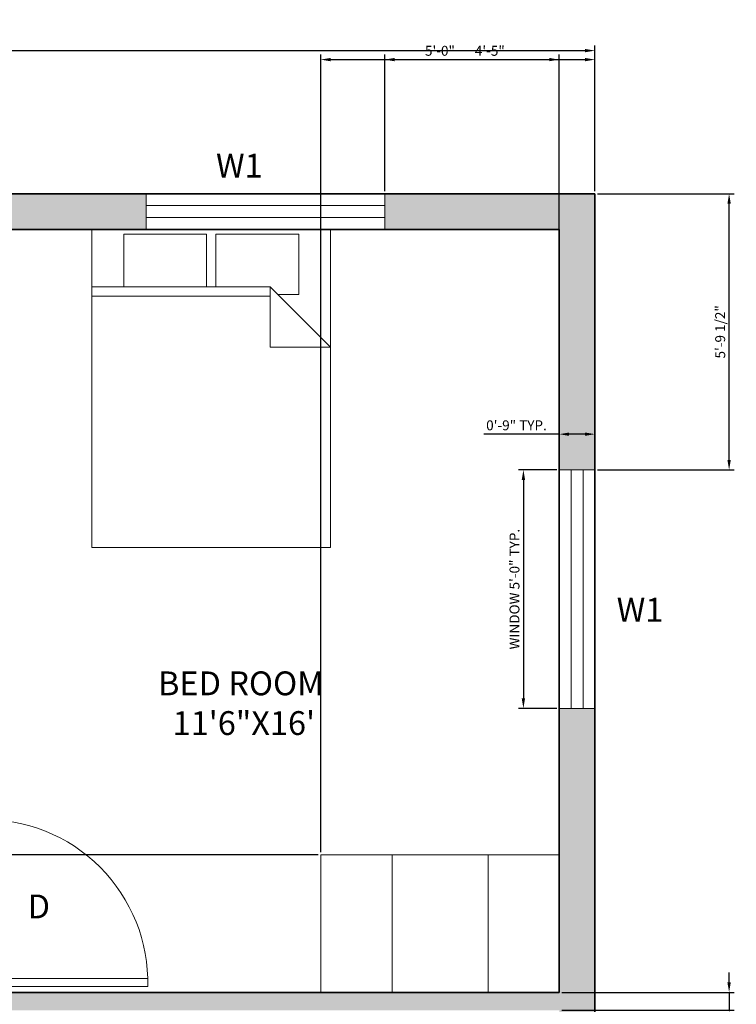
# Model space of a CAD drawing. Units: inches. Extents: x 5030 to 5465, y 5339 to 6047.
# Tile 5 of 5: x 5285 to 5465, y 5771 to 6018. Entities that reach past the tile are written whole.
import ezdxf

# ---------------------------------------------------------------- set-up
doc = ezdxf.new("R2010")
doc.units = ezdxf.units.IN
for name, color, linetype, lineweight in [('A-ANNO-DIMS', 2, 'Continuous', 18), ('A-ANNO-TEXT', 7, 'Continuous', 18), ('A-AREA-IDEN', 7, 'Continuous', 25), ('A-DOOR', 3, 'Continuous', 18), ('A-FLOR-CASE', 8, 'Continuous', 18), ('A-FURN', 8, 'Continuous', 18), ('A-GLAZ', 4, 'Continuous', 18), ('A-WALL', 7, 'Continuous', 35)]:
    doc.layers.add(name, color=color, linetype=linetype, lineweight=lineweight)
doc.layers.add('A-WALL-PATT', color=149, linetype='Continuous', lineweight=13, true_color=0x444546)
doc.styles.get("Standard").update_dxf_attribs({"font": 'arial.ttf'})
doc.dimstyles.new('ISO-25', dxfattribs={"dimtxt": 2.5, "dimasz": 2.5, "dimexe": 1.25, "dimexo": 0.625, "dimtad": 1, "dimlunit": 3, "dimtxsty": 'Standard', "dimcen": 2.5, "dimadec": 0, "dimazin": 0, "dimtfac": 1, "dimtmove": 0, "dimatfit": 3, "dimfxl": 1, "dimarcsym": 0})

# ---------------------------------------------------------------- blocks, each defined once
blk = doc.blocks.new('Bed - Queen')
for p, q in [((0, -80.00003), (0, 0)), ((0, 0), (59.99999, 0)), ((59.99999, 0), (59.99999, -80.00003)), ((7.99999, -1.2), (28.79998, -1.2)), ((7.99999, -14.4), (7.99999, -1.2)), ((28.79998, -1.2), (28.79998, -14.4)), ((31.19999, -1.2), (51.99999, -1.2)), ((31.19999, -14.4), (31.19999, -1.2)), ((51.99999, -1.2), (51.99999, -16.4)), ((0, -14.4), (44.8, -14.4)), ((59.99999, -29.6), (44.8, -14.4)), ((44.8, -14.4), (44.8, -29.6)), ((44.8, -16.8), (0, -16.8)), ((51.99999, -16.4), (46.79936, -16.4)), ((44.8, -29.6), (59.99999, -29.6)), ((59.99999, -80.00003), (0, -80.00003))]:
    blk.add_line(p, q)
blk = doc.blocks.new('*D7')
at = {"layer": 'A-ANNO-DIMS', "color": 0, "lineweight": -2, "transparency": 16777216}
for p, q in [((5069.24, 5975.13), (5069.24, 6011.77)), ((5429.24, 5975.13), (5429.24, 6011.77)), ((5071.74, 6010.52), (5426.74, 6010.52))]:
    blk.add_line(p, q, dxfattribs=at)
at = {"layer": 'A-ANNO-DIMS', "color": 0, "transparency": 16777216}
for points in [[(5071.74, 6010.94), (5071.74, 6010.1), (5069.24, 6010.52)], [(5426.74, 6010.94), (5426.74, 6010.1), (5429.24, 6010.52)]]:
    blk.add_solid(points, dxfattribs=at)
at = {"layer": 'Defpoints', "color": 0, "transparency": 16777216}
for p in [(5429.24, 6010.52), (5069.24, 5974.5), (5429.24, 5974.5)]:
    blk.add_point(p, dxfattribs=at)
at = {"layer": 'A-ANNO-DIMS', "color": 0, "transparency": 16777216, "insert": (5249.24, 6014.21), "char_height": 6, "attachment_point": 5}
blk.add_mtext("30'", dxfattribs=at)
blk = doc.blocks.new('WIN-60IN')
for p, q in [((0, 60), (9, 60)), ((3, 60), (3, 0)), ((6, 60), (6, 0)), ((0, 0), (9, 0))]:
    blk.add_line(p, q)
blk = doc.blocks.new('DOOR-SWING-42IN')
for p, q in [((0, 0), (0, 42)), ((0, 42), (2, 42)), ((2, 42), (2, 0)), ((2, 0), (0, 0))]:
    blk.add_line(p, q)
blk.add_arc((1, 1), 41.01, 358.6028, 91.3972)
blk = doc.blocks.new('*D13')
at = {"layer": 'A-ANNO-DIMS', "color": 0, "lineweight": -2, "transparency": 16777216}
for p, q in [((5419.62, 5904.99), (5409.99, 5904.99)), ((5411.24, 5902.49), (5411.24, 5847.49)), ((5419.62, 5844.99), (5409.99, 5844.99))]:
    blk.add_line(p, q, dxfattribs=at)
at = {"layer": 'A-ANNO-DIMS', "color": 0, "transparency": 16777216}
for points in [[(5410.82, 5902.49), (5411.66, 5902.49), (5411.24, 5904.99)], [(5410.82, 5847.49), (5411.66, 5847.49), (5411.24, 5844.99)]]:
    blk.add_solid(points, dxfattribs=at)
at = {"layer": 'Defpoints', "color": 0, "transparency": 16777216}
for p in [(5420.24, 5904.99), (5411.24, 5844.99), (5420.24, 5844.99)]:
    blk.add_point(p, dxfattribs=at)
at = {"layer": 'A-ANNO-DIMS', "color": 0, "transparency": 16777216, "insert": (5409.32, 5874.99), "char_height": 2.5, "attachment_point": 5, "rotation": 90}
blk.add_mtext('WINDOW 5\'-0" TYP.', dxfattribs=at)
blk = doc.blocks.new('*D14')
at = {"layer": 'A-ANNO-DIMS', "color": 0, "lineweight": -2, "transparency": 16777216}
for p, q in [((5420.24, 5905.61), (5420.24, 5915.24)), ((5429.24, 5905.61), (5429.24, 5915.24)), ((5420.24, 5913.99), (5401.25, 5913.99)), ((5426.74, 5913.99), (5422.74, 5913.99))]:
    blk.add_line(p, q, dxfattribs=at)
at = {"layer": 'A-ANNO-DIMS', "color": 0, "transparency": 16777216}
for points in [[(5422.74, 5914.4), (5422.74, 5913.57), (5420.24, 5913.99)], [(5426.74, 5914.4), (5426.74, 5913.57), (5429.24, 5913.99)]]:
    blk.add_solid(points, dxfattribs=at)
at = {"layer": 'Defpoints', "color": 0, "transparency": 16777216}
for p in [(5420.24, 5913.99), (5420.24, 5904.99), (5429.24, 5904.99)]:
    blk.add_point(p, dxfattribs=at)
at = {"layer": 'A-ANNO-DIMS', "color": 0, "transparency": 16777216, "insert": (5409.5, 5915.89), "char_height": 2.5, "attachment_point": 5}
blk.add_mtext('0\'-9" TYP.', dxfattribs=at)
blk = doc.blocks.new('*D42')
at = {"layer": 'A-ANNO-DIMS', "color": 0, "lineweight": -2, "transparency": 16777216}
for p, q in [((5429.87, 5974.5), (5464.24, 5974.5)), ((5462.99, 5907.49), (5462.99, 5972)), ((5429.87, 5904.99), (5464.24, 5904.99))]:
    blk.add_line(p, q, dxfattribs=at)
at = {"layer": 'A-ANNO-DIMS', "color": 0, "transparency": 16777216}
for points in [[(5462.57, 5972), (5463.41, 5972), (5462.99, 5974.5)], [(5462.57, 5907.49), (5463.41, 5907.49), (5462.99, 5904.99)]]:
    blk.add_solid(points, dxfattribs=at)
at = {"layer": 'Defpoints', "color": 0, "transparency": 16777216}
for p in [(5429.24, 5974.5), (5462.99, 5974.5), (5429.24, 5904.99)]:
    blk.add_point(p, dxfattribs=at)
at = {"layer": 'A-ANNO-DIMS', "color": 0, "transparency": 16777216, "insert": (5461.07, 5939.74), "char_height": 2.5, "attachment_point": 5, "rotation": 90}
blk.add_mtext('5\'-9 1/2"', dxfattribs=at)
blk = doc.blocks.new('*D43')
at = {"layer": 'A-ANNO-DIMS', "color": 0, "lineweight": -2, "transparency": 16777216}
for p, q in [((5376.34, 5975.13), (5376.34, 6009.5)), ((5429.24, 5975.13), (5429.24, 6009.5)), ((5378.84, 6008.25), (5426.74, 6008.25))]:
    blk.add_line(p, q, dxfattribs=at)
at = {"layer": 'A-ANNO-DIMS', "color": 0, "transparency": 16777216}
for points in [[(5378.84, 6008.67), (5378.84, 6007.84), (5376.34, 6008.25)], [(5426.74, 6008.67), (5426.74, 6007.84), (5429.24, 6008.25)]]:
    blk.add_solid(points, dxfattribs=at)
at = {"layer": 'Defpoints', "color": 0, "transparency": 16777216}
for p in [(5429.24, 6008.25), (5376.34, 5974.5), (5429.24, 5974.5)]:
    blk.add_point(p, dxfattribs=at)
at = {"layer": 'A-ANNO-DIMS', "color": 0, "transparency": 16777216, "insert": (5402.79, 6010.15), "char_height": 2.5, "attachment_point": 5}
blk.add_mtext('4\'-5"', dxfattribs=at)
blk = doc.blocks.new('*D56')
at = {"layer": 'A-ANNO-DIMS', "color": 0, "lineweight": -2, "transparency": 16777216}
for p, q in [((5360.24, 5808.77), (5360.24, 6009.5)), ((5420.24, 5808.77), (5420.24, 6009.5)), ((5362.74, 6008.25), (5417.74, 6008.25))]:
    blk.add_line(p, q, dxfattribs=at)
at = {"layer": 'A-ANNO-DIMS', "color": 0, "transparency": 16777216}
for points in [[(5362.74, 6008.67), (5362.74, 6007.84), (5360.24, 6008.25)], [(5417.74, 6008.67), (5417.74, 6007.84), (5420.24, 6008.25)]]:
    blk.add_solid(points, dxfattribs=at)
at = {"layer": 'Defpoints', "color": 0, "transparency": 16777216}
for p in [(5420.24, 6008.25), (5360.24, 5808.14), (5420.24, 5808.14)]:
    blk.add_point(p, dxfattribs=at)
at = {"layer": 'A-ANNO-DIMS', "color": 0, "transparency": 16777216, "insert": (5390.24, 6010.15), "char_height": 2.5, "attachment_point": 5}
blk.add_mtext('5\'-0"', dxfattribs=at)
blk = doc.blocks.new('*D57')
at = {"layer": 'A-ANNO-DIMS', "color": 0, "lineweight": -2, "transparency": 16777216}
for p, q in [((5359.62, 5808.14), (5034.24, 5808.14)), ((5035.49, 5776), (5035.49, 5805.64)), ((5359.62, 5773.5), (5034.24, 5773.5))]:
    blk.add_line(p, q, dxfattribs=at)
at = {"layer": 'A-ANNO-DIMS', "color": 0, "transparency": 16777216}
for points in [[(5035.07, 5805.64), (5035.91, 5805.64), (5035.49, 5808.14)], [(5035.07, 5776), (5035.91, 5776), (5035.49, 5773.5)]]:
    blk.add_solid(points, dxfattribs=at)
at = {"layer": 'Defpoints', "color": 0, "transparency": 16777216}
for p in [(5035.49, 5808.14), (5360.24, 5808.14), (5360.24, 5773.5)]:
    blk.add_point(p, dxfattribs=at)
at = {"layer": 'A-ANNO-DIMS', "color": 0, "transparency": 16777216, "insert": (5033.57, 5790.82), "char_height": 2.5, "attachment_point": 5, "rotation": 90}
blk.add_mtext('2\'-10 1/2"', dxfattribs=at)
blk = doc.blocks.new('*D62')
at = {"layer": 'A-ANNO-DIMS', "color": 0, "lineweight": -2, "transparency": 16777216}
for p, q in [((5462.99, 5776), (5462.99, 5778.5)), ((5420.87, 5773.5), (5464.24, 5773.5)), ((5462.99, 5773.5), (5462.99, 5769)), ((5420.87, 5769), (5464.24, 5769)), ((5462.99, 5766.5), (5462.99, 5750.28))]:
    blk.add_line(p, q, dxfattribs=at)
at = {"layer": 'A-ANNO-DIMS', "color": 0, "transparency": 16777216}
for points in [[(5462.57, 5776), (5463.41, 5776), (5462.99, 5773.5)], [(5462.57, 5766.5), (5463.41, 5766.5), (5462.99, 5769)]]:
    blk.add_solid(points, dxfattribs=at)
at = {"layer": 'Defpoints', "color": 0, "transparency": 16777216}
for p in [(5420.24, 5773.5), (5420.24, 5769), (5462.99, 5769)]:
    blk.add_point(p, dxfattribs=at)
at = {"layer": 'A-ANNO-DIMS', "color": 0, "transparency": 16777216, "insert": (5461.07, 5757.14), "char_height": 2.5, "attachment_point": 5, "rotation": 90}
blk.add_mtext('0\'-4 1/2"', dxfattribs=at)

msp = doc.modelspace()

# ---------------------------------------------------------------- hatches: boundary and pattern name
at = {"layer": 'A-WALL-PATT'}
h = msp.add_hatch(color=256, dxfattribs=at)
h.dxf.hatch_style = 1
h.paths.add_polyline_path([(5227.999, 5974.503), (5069.24, 5974.503), (5069.24, 5942.38), (5078.24, 5942.38), (5078.24, 5965.503), (5198.24, 5965.503), (5198.24, 5916.003), (5274.74, 5916.003), (5274.74, 5869.503), (5202.74, 5869.503), (5202.74, 5898.003), (5198.24, 5898.003), (5198.24, 5865.003), (5274.74, 5865.003), (5274.74, 5817.003, -0.0121933), (5276.74, 5817.003), (5279.24, 5817.003), (5279.24, 5947.503, -0.0293864), (5277.24, 5947.503), (5274.74, 5947.503), (5274.74, 5920.503), (5202.74, 5920.503), (5202.74, 5965.503), (5227.999, 5965.503)])
h.paths.add_polyline_path([(5078.24, 5894.38), (5069.24, 5894.38), (5069.24, 5845.837), (5078.24, 5845.837), (5078.24, 5865.003), (5138.24, 5865.003), (5138.24, 5869.503), (5078.24, 5869.503)], flags=17)
h.paths.add_polyline_path([(5316.341, 5974.503), (5251.999, 5974.503), (5251.999, 5965.503), (5279.24, 5965.503), (5316.341, 5965.503)])
h.paths.add_polyline_path([(5429.24, 5974.503), (5376.341, 5974.503), (5376.341, 5965.503), (5420.24, 5965.503), (5420.24, 5904.986), (5429.24, 5904.986)])
h.paths.add_polyline_path([(5429.24, 5844.986), (5420.24, 5844.986), (5420.24, 5773.503), (5279.24, 5773.503), (5279.24, 5775.003), (5274.74, 5775.003), (5274.74, 5644.503), (5279.24, 5644.503), (5279.24, 5686.503), (5279.24, 5769.003), (5420.24, 5769.003), (5420.24, 5738.095), (5429.24, 5738.095)])
h.paths.add_polyline_path([(5429.24, 5678.095), (5420.24, 5678.095), (5420.24, 5649.003), (5321.24, 5649.003), (5321.24, 5646.503, -0.0121933), (5321.24, 5644.503), (5343.74, 5644.503), (5343.74, 5614.503, -0.0293864), (5345.74, 5614.503), (5348.24, 5614.503), (5348.24, 5644.503), (5420.24, 5644.503), (5420.24, 5636.807), (5429.24, 5636.807)])
h.paths.add_polyline_path([(5429.24, 5612.807), (5420.24, 5612.807), (5420.24, 5596.503), (5321.24, 5596.503, -0.0121933), (5321.24, 5594.503), (5321.24, 5592.003), (5420.24, 5592.003), (5420.24, 5566.431), (5429.24, 5566.431)])
h.paths.add_polyline_path([(5429.24, 5506.431), (5420.24, 5506.431), (5420.24, 5472.003), (5279.24, 5472.003), (5279.24, 5596.503), (5126.24, 5596.503), (5126.24, 5589.503, -0.0106371), (5126.24, 5587.503), (5274.74, 5587.503), (5274.74, 5468.003), (5420.24, 5468.003), (5420.24, 5452.536), (5429.24, 5452.536)])
h.paths.add_polyline_path([(5429.24, 5392.536), (5420.24, 5392.536), (5420.24, 5383.503), (5274.74, 5383.503), (5274.74, 5374.503), (5429.24, 5374.503)])
h.paths.add_polyline_path([(5101.667, 5383.503), (5078.24, 5383.503), (5078.24, 5683.152), (5069.24, 5683.152), (5069.24, 5374.503), (5101.667, 5374.503)])
h.paths.add_polyline_path([(5078.24, 5770.503), (5221.745, 5770.503), (5221.745, 5775.003), (5078.24, 5775.003), (5078.24, 5785.837), (5069.24, 5785.837), (5069.24, 5743.152), (5078.24, 5743.152)])
h.paths.add_polyline_path([(5274.74, 5379.003), (5101.667, 5379.003), (5101.667, 5374.503), (5274.74, 5374.503)])

# ---------------------------------------------------------------- linework, layer by layer
at = {"layer": 'A-FLOR-CASE'}
for p, q in [((5372.24, 5808.145), (5360.24, 5808.145)), ((5360.24, 5808.145), (5360.24, 5773.503)), ((5360.24, 5808.145), (5372.24, 5808.145)), ((5420.24, 5808.145), (5372.24, 5808.145)), ((5378.24, 5808.145), (5378.24, 5773.503)), ((5402.393, 5808.145), (5402.393, 5773.503))]:
    msp.add_line(p, q, dxfattribs=at)
at = {"layer": 'A-WALL'}
for p, q in [((5069.24, 5974.503), (5429.24, 5974.503)), ((5429.24, 5974.503), (5429.24, 5374.503)), ((5279.24, 5965.503), (5420.24, 5965.503)), ((5420.24, 5965.503), (5420.24, 5773.503)), ((5279.24, 5773.503), (5420.24, 5773.503))]:
    msp.add_line(p, q, dxfattribs=at)

# ---------------------------------------------------------------- block references
at = {"layer": 'A-DOOR', "extrusion": (0, 0, -1), "zscale": -1, "rotation": 90.00000000000831}
msp.add_blockref('DOOR-SWING-42IN', (-5274.74, 5775.003), dxfattribs=at)
at = {"layer": 'A-FURN'}
msp.add_blockref('Bed - Queen', (5302.702, 5965.503), dxfattribs=at)
at = {"layer": 'A-GLAZ'}
for p, rotation in [((5316.341, 5974.503), 270.0000000000034), ((5429.24, 5904.986), 180)]:
    msp.add_blockref('WIN-60IN', p, dxfattribs=dict(at, rotation=rotation))

# ---------------------------------------------------------------- texts
at = {"layer": 'A-ANNO-TEXT', "char_height": 6, "attachment_point": 1}
for s, insert in [('   W1  ', (5328.409, 5984.576)), ('W1', (5434.716, 5872.807)), ('D', (5286.512, 5798.136))]:
    msp.add_mtext_dynamic_manual_height_columns(s, width=54.21026, gutter_width=12.5, heights=[0], dxfattribs=dict(at, insert=insert))
at = {"layer": 'A-AREA-IDEN', "insert": (5317.491, 5854.277), "char_height": 6, "attachment_point": 1}
msp.add_mtext_dynamic_manual_height_columns(' BED ROOM\\P   11\'6"X16\'', width=54.21026, gutter_width=12.5, heights=[0], dxfattribs=at)

# ---------------------------------------------------------------- dimensions: what is measured, and where the dimension line sits
at = {"layer": 'A-ANNO-DIMS'}
for base, p1, p2, override, picture, middle in [((5429.24, 6010.52), (5069.24, 5974.503), (5429.24, 5974.503), {"dimtxt": 6, "dimclrd": 0, "dimclre": 0, "dimclrt": 0}, '*D7', (5249.24, 6014.211)), ((5420.24, 6008.253), (5360.24, 5808.145), (5420.24, 5808.145), {"dimdec": 1, "dimlfac": 1, "dimrnd": 0, "dimzin": 1, "dimdsep": 46, "dimlunit": 4, "dimfrac": 2}, '*D56', (5390.24, 6010.155)), ((5429.24, 6008.253), (5376.341, 5974.503), (5429.24, 5974.503), {"dimdec": 1, "dimlfac": 1, "dimrnd": 0, "dimzin": 1, "dimdsep": 46, "dimlunit": 4, "dimfrac": 2}, '*D43', (5402.791, 6010.149))]:
    dim = msp.add_linear_dim(base=base, p1=p1, p2=p2, dimstyle='ISO-25', override=override, dxfattribs=at)
    dim.commit()
    dim.dimension.update_dxf_attribs({"geometry": picture, "text_midpoint": middle})
for base, p1, p2, picture, middle in [((5462.99, 5974.503), (5429.24, 5904.986), (5429.24, 5974.503), '*D42', (5461.073, 5939.745)), ((5035.49, 5808.145), (5360.24, 5773.503), (5360.24, 5808.145), '*D57', (5033.573, 5790.824)), ((5462.99, 5769.003), (5420.24, 5773.503), (5420.24, 5769.003), '*D62', (5461.073, 5757.143))]:
    dim = msp.add_linear_dim(base=base, p1=p1, p2=p2, angle=90, dimstyle='ISO-25', override={"dimdec": 1, "dimlfac": 1, "dimrnd": 0, "dimzin": 1, "dimdsep": 46, "dimlunit": 4, "dimfrac": 2}, dxfattribs=at)
    dim.commit()
    dim.dimension.update_dxf_attribs({"geometry": picture, "text_midpoint": middle})
for base, p1, p2, angle, text, picture, middle in [((5420.24, 5913.986), (5429.24, 5904.986), (5420.24, 5904.986), 180, '<> TYP.', '*D14', (5409.496, 5915.888)), ((5411.24, 5844.986), (5420.24, 5904.986), (5420.24, 5844.986), 270, 'WINDOW <> TYP.', '*D13', (5409.322, 5874.986))]:
    dim = msp.add_linear_dim(base=base, p1=p1, p2=p2, angle=angle, text=text, dimstyle='ISO-25', override={"dimdec": 1, "dimlfac": 1, "dimrnd": 0, "dimzin": 1, "dimdsep": 46, "dimlunit": 4, "dimfrac": 2}, dxfattribs=at)
    dim.commit()
    dim.dimension.update_dxf_attribs({"geometry": picture, "text_midpoint": middle})

doc.saveas('drawing.dxf')
